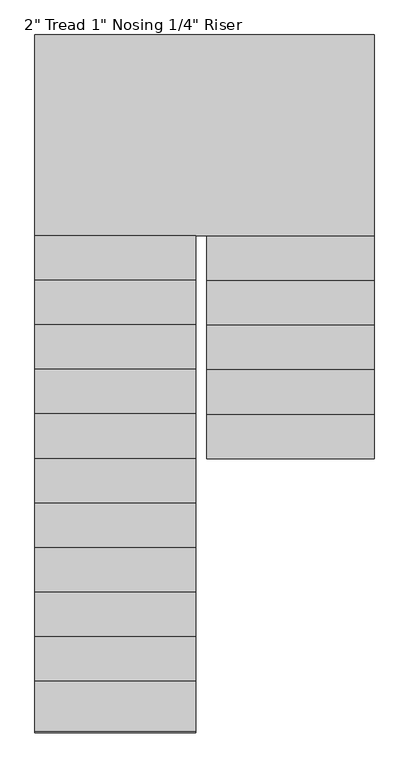
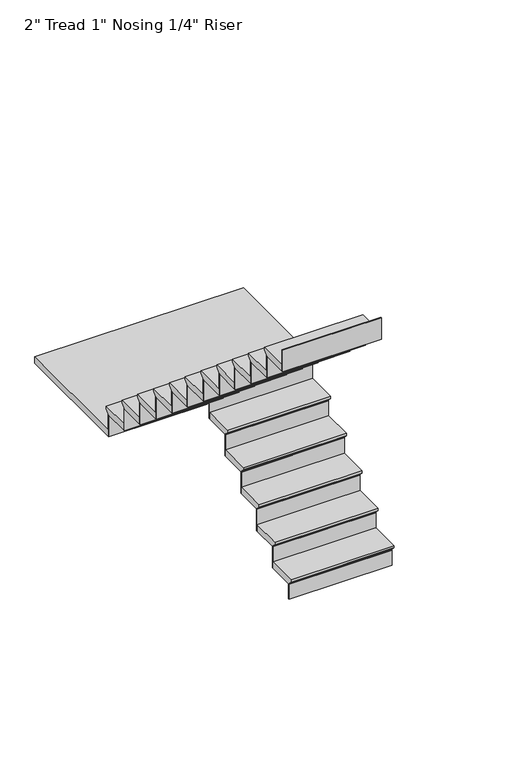
"""IFC4 building model written with IfcOpenShell, lengths in millimetres: stair flight geometry."""

from ifc_helpers import new_model, si_unit, origin, place, context, project, spatial, faceted_brep, source, transform, mapped, element, save


def stair_flight_8b765581(model_context):
    return source(origin(), model_context, "Body", "Brep", [
        faceted_brep([(-3749.597125, 2714.6319226, 33525.8833333), (-3749.597125, 2714.6319226, 33544.9333333), (-4512.2136682, 2714.6319226, 33544.9333333), (-4512.2136682, 2714.6319226, 33525.8833333), (-3749.597125, 2740.0319226, 33500.4833333), (-4512.2136682, 2740.0319226, 33500.4833333), (-3749.597125, 2943.2319226, 33544.9333333), (-4512.2136682, 2943.2319226, 33544.9333333), (-4512.2136682, 2740.0319226, 33494.1333333), (-4512.2136682, 2943.2319226, 33494.1333333), (-3749.597125, 2943.2319226, 33494.1333333), (-3749.597125, 2740.0319226, 33494.1333333)], [[[0, 1, 2, 3]], [[4, 0, 3, 5]], [[2, 1, 6, 7]], [[8, 9, 10, 11]], [[2, 7, 9, 8, 5, 3]], [[8, 11, 4, 5]], [[6, 1, 0, 4, 11, 10]], [[7, 6, 10, 9]]]),
        faceted_brep([(-3749.597125, 2740.0319226, 33494.1333333), (-3749.597125, 2740.0319226, 33375.6), (-3749.597125, 2746.3819226, 33375.6), (-3749.597125, 2746.3819226, 33494.1333333), (-4512.2136682, 2740.0319226, 33494.1333333), (-4512.2136682, 2746.3819226, 33494.1333333), (-4512.2136682, 2746.3819226, 33375.6), (-4512.2136682, 2740.0319226, 33375.6)], [[[0, 1, 2, 3]], [[4, 5, 6, 7]], [[1, 0, 4, 7]], [[2, 1, 7, 6]], [[3, 2, 6, 5]], [[0, 3, 5, 4]]]),
        faceted_brep([(-3749.597125, 2943.2319226, 33663.4666667), (-3749.597125, 2943.2319226, 33494.1333333), (-3749.597125, 2949.5819226, 33494.1333333), (-3749.597125, 2949.5819226, 33663.4666667), (-4512.2136682, 2943.2319226, 33663.4666667), (-4512.2136682, 2949.5819226, 33663.4666667), (-4512.2136682, 2949.5819226, 33494.1333333), (-4512.2136682, 2943.2319226, 33494.1333333)], [[[0, 1, 2, 3]], [[4, 5, 6, 7]], [[1, 0, 4, 7]], [[2, 1, 7, 6]], [[3, 2, 6, 5]], [[0, 3, 5, 4]]]),
        faceted_brep([(-4512.2136682, 2917.8319226, 33714.2666667), (-3749.597125, 2917.8319226, 33714.2666667), (-3749.597125, 3146.4319226, 33714.2666667), (-4512.2136682, 3146.4319226, 33714.2666667), (-4512.2136682, 2943.2319226, 33663.4666667), (-4512.2136682, 3146.4319226, 33663.4666667), (-3749.597125, 3146.4319226, 33663.4666667), (-3749.597125, 2943.2319226, 33663.4666667), (-4512.2136682, 2943.2319226, 33669.8166667), (-4512.2136682, 2917.8319226, 33695.2166667), (-3749.597125, 2943.2319226, 33669.8166667), (-3749.597125, 2917.8319226, 33695.2166667)], [[[0, 1, 2, 3]], [[4, 5, 6, 7]], [[0, 3, 5, 4, 8, 9]], [[4, 7, 10, 8]], [[2, 1, 11, 10, 7, 6]], [[3, 2, 6, 5]], [[11, 1, 0, 9]], [[10, 11, 9, 8]]]),
        faceted_brep([(-3749.597125, 3146.4319226, 33832.8), (-3749.597125, 3146.4319226, 33663.4666667), (-3749.597125, 3152.7819226, 33663.4666667), (-3749.597125, 3152.7819226, 33832.8), (-4512.2136682, 3146.4319226, 33832.8), (-4512.2136682, 3152.7819226, 33832.8), (-4512.2136682, 3152.7819226, 33663.4666667), (-4512.2136682, 3146.4319226, 33663.4666667)], [[[0, 1, 2, 3]], [[4, 5, 6, 7]], [[1, 0, 4, 7]], [[2, 1, 7, 6]], [[3, 2, 6, 5]], [[0, 3, 5, 4]]]),
        faceted_brep([(-4512.2136682, 3121.0319226, 33883.6), (-3749.597125, 3121.0319226, 33883.6), (-3749.597125, 3349.6319226, 33883.6), (-4512.2136682, 3349.6319226, 33883.6), (-4512.2136682, 3146.4319226, 33832.8), (-4512.2136682, 3349.6319226, 33832.8), (-3749.597125, 3349.6319226, 33832.8), (-3749.597125, 3146.4319226, 33832.8), (-4512.2136682, 3146.4319226, 33839.15), (-4512.2136682, 3121.0319226, 33864.55), (-3749.597125, 3146.4319226, 33839.15), (-3749.597125, 3121.0319226, 33864.55)], [[[0, 1, 2, 3]], [[4, 5, 6, 7]], [[0, 3, 5, 4, 8, 9]], [[4, 7, 10, 8]], [[2, 1, 11, 10, 7, 6]], [[3, 2, 6, 5]], [[11, 1, 0, 9]], [[10, 11, 9, 8]]]),
        faceted_brep([(-3749.597125, 3349.6319226, 34002.1333333), (-3749.597125, 3349.6319226, 33832.8), (-3749.597125, 3355.9819226, 33832.8), (-3749.597125, 3355.9819226, 34002.1333333), (-4512.2136682, 3349.6319226, 34002.1333333), (-4512.2136682, 3355.9819226, 34002.1333333), (-4512.2136682, 3355.9819226, 33832.8), (-4512.2136682, 3349.6319226, 33832.8)], [[[0, 1, 2, 3]], [[4, 5, 6, 7]], [[1, 0, 4, 7]], [[2, 1, 7, 6]], [[3, 2, 6, 5]], [[0, 3, 5, 4]]]),
        faceted_brep([(-4512.2136682, 3324.2319226, 34052.9333333), (-3749.597125, 3324.2319226, 34052.9333333), (-3749.597125, 3552.8319226, 34052.9333333), (-4512.2136682, 3552.8319226, 34052.9333333), (-4512.2136682, 3349.6319226, 34002.1333333), (-4512.2136682, 3552.8319226, 34002.1333333), (-3749.597125, 3552.8319226, 34002.1333333), (-3749.597125, 3349.6319226, 34002.1333333), (-4512.2136682, 3349.6319226, 34008.4833333), (-4512.2136682, 3324.2319226, 34033.8833333), (-3749.597125, 3349.6319226, 34008.4833333), (-3749.597125, 3324.2319226, 34033.8833333)], [[[0, 1, 2, 3]], [[4, 5, 6, 7]], [[0, 3, 5, 4, 8, 9]], [[4, 7, 10, 8]], [[2, 1, 11, 10, 7, 6]], [[3, 2, 6, 5]], [[11, 1, 0, 9]], [[10, 11, 9, 8]]]),
        faceted_brep([(-3749.597125, 3552.8319226, 34171.4666667), (-3749.597125, 3552.8319226, 34002.1333333), (-3749.597125, 3559.1819226, 34002.1333333), (-3749.597125, 3559.1819226, 34171.4666667), (-4512.2136682, 3552.8319226, 34171.4666667), (-4512.2136682, 3559.1819226, 34171.4666667), (-4512.2136682, 3559.1819226, 34002.1333333), (-4512.2136682, 3552.8319226, 34002.1333333)], [[[0, 1, 2, 3]], [[4, 5, 6, 7]], [[1, 0, 4, 7]], [[2, 1, 7, 6]], [[3, 2, 6, 5]], [[0, 3, 5, 4]]]),
        faceted_brep([(-4512.2136682, 3527.4319226, 34222.2666667), (-3749.597125, 3527.4319226, 34222.2666667), (-3749.597125, 3756.0319226, 34222.2666667), (-4512.2136682, 3756.0319226, 34222.2666667), (-4512.2136682, 3552.8319226, 34171.4666667), (-4512.2136682, 3756.0319226, 34171.4666667), (-3749.597125, 3756.0319226, 34171.4666667), (-3749.597125, 3552.8319226, 34171.4666667), (-4512.2136682, 3552.8319226, 34177.8166667), (-4512.2136682, 3527.4319226, 34203.2166667), (-3749.597125, 3552.8319226, 34177.8166667), (-3749.597125, 3527.4319226, 34203.2166667)], [[[0, 1, 2, 3]], [[4, 5, 6, 7]], [[0, 3, 5, 4, 8, 9]], [[4, 7, 10, 8]], [[2, 1, 11, 10, 7, 6]], [[3, 2, 6, 5]], [[11, 1, 0, 9]], [[10, 11, 9, 8]]]),
        faceted_brep([(-3749.597125, 3756.0319226, 34340.8), (-3749.597125, 3756.0319226, 34171.4666667), (-3749.597125, 3762.3819226, 34171.4666667), (-3749.597125, 3762.3819226, 34340.8), (-4512.2136682, 3756.0319226, 34340.8), (-4512.2136682, 3762.3819226, 34340.8), (-4512.2136682, 3762.3819226, 34171.4666667), (-4512.2136682, 3756.0319226, 34171.4666667)], [[[0, 1, 2, 3]], [[4, 5, 6, 7]], [[1, 0, 4, 7]], [[2, 1, 7, 6]], [[3, 2, 6, 5]], [[0, 3, 5, 4]]]),
        faceted_brep([(-4563.0136682, 3705.2319226, 34391.6), (-4563.0136682, 3730.6319226, 34391.6), (-3749.597125, 3730.6319226, 34391.6), (-3749.597125, 4645.0319226, 34391.6), (-5295.0246464, 4645.0319226, 34391.6), (-5295.0246464, 3705.2319226, 34391.6), (-4563.0136682, 3730.6319226, 34340.8), (-4563.0136682, 3705.2319226, 34340.8), (-5295.0246464, 3705.2319226, 34340.8), (-5295.0246464, 4645.0319226, 34340.8), (-3749.597125, 4645.0319226, 34340.8), (-3749.597125, 3756.0319226, 34340.8), (-4512.2136682, 3756.0319226, 34340.8), (-4512.2136682, 3730.6319226, 34340.8), (-4512.2136682, 3730.6319226, 34372.55), (-3749.597125, 3730.6319226, 34372.55), (-4512.2136682, 3756.0319226, 34347.15), (-3749.597125, 3756.0319226, 34347.15)], [[[0, 1, 2, 3, 4, 5]], [[6, 7, 8, 9, 10, 11, 12, 13]], [[1, 0, 7, 6]], [[2, 1, 6, 13, 14, 15]], [[13, 12, 16, 14]], [[12, 11, 17, 16]], [[3, 2, 15, 17, 11, 10]], [[4, 3, 10, 9]], [[5, 4, 9, 8]], [[0, 5, 8, 7]], [[17, 15, 14, 16]]]),
        faceted_brep([(-5295.0246464, 3705.2319226, 34510.1333333), (-5295.0246464, 3705.2319226, 34340.8), (-5295.0246464, 3698.8819226, 34340.8), (-5295.0246464, 3698.8819226, 34510.1333333), (-4563.0136682, 3705.2319226, 34510.1333333), (-4563.0136682, 3698.8819226, 34510.1333333), (-4563.0136682, 3698.8819226, 34340.8), (-4563.0136682, 3705.2319226, 34340.8)], [[[0, 1, 2, 3]], [[4, 5, 6, 7]], [[1, 0, 4, 7]], [[2, 1, 7, 6]], [[3, 2, 6, 5]], [[0, 3, 5, 4]]]),
        faceted_brep([(-4563.0136682, 3730.6319226, 34560.9333333), (-5295.0246464, 3730.6319226, 34560.9333333), (-5295.0246464, 3502.0319226, 34560.9333333), (-4563.0136682, 3502.0319226, 34560.9333333), (-4563.0136682, 3705.2319226, 34510.1333333), (-4563.0136682, 3502.0319226, 34510.1333333), (-5295.0246464, 3502.0319226, 34510.1333333), (-5295.0246464, 3705.2319226, 34510.1333333), (-4563.0136682, 3705.2319226, 34516.4833333), (-4563.0136682, 3730.6319226, 34541.8833333), (-5295.0246464, 3705.2319226, 34516.4833333), (-5295.0246464, 3730.6319226, 34541.8833333)], [[[0, 1, 2, 3]], [[4, 5, 6, 7]], [[0, 3, 5, 4, 8, 9]], [[4, 7, 10, 8]], [[2, 1, 11, 10, 7, 6]], [[3, 2, 6, 5]], [[11, 1, 0, 9]], [[10, 11, 9, 8]]]),
        faceted_brep([(-5295.0246464, 3502.0319226, 34679.4666667), (-5295.0246464, 3502.0319226, 34510.1333333), (-5295.0246464, 3495.6819226, 34510.1333333), (-5295.0246464, 3495.6819226, 34679.4666667), (-4563.0136682, 3502.0319226, 34679.4666667), (-4563.0136682, 3495.6819226, 34679.4666667), (-4563.0136682, 3495.6819226, 34510.1333333), (-4563.0136682, 3502.0319226, 34510.1333333)], [[[0, 1, 2, 3]], [[4, 5, 6, 7]], [[1, 0, 4, 7]], [[2, 1, 7, 6]], [[3, 2, 6, 5]], [[0, 3, 5, 4]]]),
        faceted_brep([(-4563.0136682, 3527.4319226, 34730.2666667), (-5295.0246464, 3527.4319226, 34730.2666667), (-5295.0246464, 3298.8319226, 34730.2666667), (-4563.0136682, 3298.8319226, 34730.2666667), (-4563.0136682, 3502.0319226, 34679.4666667), (-4563.0136682, 3298.8319226, 34679.4666667), (-5295.0246464, 3298.8319226, 34679.4666667), (-5295.0246464, 3502.0319226, 34679.4666667), (-4563.0136682, 3502.0319226, 34685.8166667), (-4563.0136682, 3527.4319226, 34711.2166667), (-5295.0246464, 3502.0319226, 34685.8166667), (-5295.0246464, 3527.4319226, 34711.2166667)], [[[0, 1, 2, 3]], [[4, 5, 6, 7]], [[0, 3, 5, 4, 8, 9]], [[4, 7, 10, 8]], [[2, 1, 11, 10, 7, 6]], [[3, 2, 6, 5]], [[11, 1, 0, 9]], [[10, 11, 9, 8]]]),
        faceted_brep([(-5295.0246464, 3298.8319226, 34848.8), (-5295.0246464, 3298.8319226, 34679.4666667), (-5295.0246464, 3292.4819226, 34679.4666667), (-5295.0246464, 3292.4819226, 34848.8), (-4563.0136682, 3298.8319226, 34848.8), (-4563.0136682, 3292.4819226, 34848.8), (-4563.0136682, 3292.4819226, 34679.4666667), (-4563.0136682, 3298.8319226, 34679.4666667)], [[[0, 1, 2, 3]], [[4, 5, 6, 7]], [[1, 0, 4, 7]], [[2, 1, 7, 6]], [[3, 2, 6, 5]], [[0, 3, 5, 4]]]),
        faceted_brep([(-4563.0136682, 3324.2319226, 34899.6), (-5295.0246464, 3324.2319226, 34899.6), (-5295.0246464, 3095.6319226, 34899.6), (-4563.0136682, 3095.6319226, 34899.6), (-4563.0136682, 3298.8319226, 34848.8), (-4563.0136682, 3095.6319226, 34848.8), (-5295.0246464, 3095.6319226, 34848.8), (-5295.0246464, 3298.8319226, 34848.8), (-4563.0136682, 3298.8319226, 34855.15), (-4563.0136682, 3324.2319226, 34880.55), (-5295.0246464, 3298.8319226, 34855.15), (-5295.0246464, 3324.2319226, 34880.55)], [[[0, 1, 2, 3]], [[4, 5, 6, 7]], [[0, 3, 5, 4, 8, 9]], [[4, 7, 10, 8]], [[2, 1, 11, 10, 7, 6]], [[3, 2, 6, 5]], [[11, 1, 0, 9]], [[10, 11, 9, 8]]]),
        faceted_brep([(-5295.0246464, 3095.6319226, 35018.1333333), (-5295.0246464, 3095.6319226, 34848.8), (-5295.0246464, 3089.2819226, 34848.8), (-5295.0246464, 3089.2819226, 35018.1333333), (-4563.0136682, 3095.6319226, 35018.1333333), (-4563.0136682, 3089.2819226, 35018.1333333), (-4563.0136682, 3089.2819226, 34848.8), (-4563.0136682, 3095.6319226, 34848.8)], [[[0, 1, 2, 3]], [[4, 5, 6, 7]], [[1, 0, 4, 7]], [[2, 1, 7, 6]], [[3, 2, 6, 5]], [[0, 3, 5, 4]]]),
        faceted_brep([(-4563.0136682, 3121.0319226, 35068.9333333), (-5295.0246464, 3121.0319226, 35068.9333333), (-5295.0246464, 2892.4319226, 35068.9333333), (-4563.0136682, 2892.4319226, 35068.9333333), (-4563.0136682, 3095.6319226, 35018.1333333), (-4563.0136682, 2892.4319226, 35018.1333333), (-5295.0246464, 2892.4319226, 35018.1333333), (-5295.0246464, 3095.6319226, 35018.1333333), (-4563.0136682, 3095.6319226, 35024.4833333), (-4563.0136682, 3121.0319226, 35049.8833333), (-5295.0246464, 3095.6319226, 35024.4833333), (-5295.0246464, 3121.0319226, 35049.8833333)], [[[0, 1, 2, 3]], [[4, 5, 6, 7]], [[0, 3, 5, 4, 8, 9]], [[4, 7, 10, 8]], [[2, 1, 11, 10, 7, 6]], [[3, 2, 6, 5]], [[11, 1, 0, 9]], [[10, 11, 9, 8]]]),
        faceted_brep([(-5295.0246464, 2892.4319226, 35187.4666667), (-5295.0246464, 2892.4319226, 35018.1333333), (-5295.0246464, 2886.0819226, 35018.1333333), (-5295.0246464, 2886.0819226, 35187.4666667), (-4563.0136682, 2892.4319226, 35187.4666667), (-4563.0136682, 2886.0819226, 35187.4666667), (-4563.0136682, 2886.0819226, 35018.1333333), (-4563.0136682, 2892.4319226, 35018.1333333)], [[[0, 1, 2, 3]], [[4, 5, 6, 7]], [[1, 0, 4, 7]], [[2, 1, 7, 6]], [[3, 2, 6, 5]], [[0, 3, 5, 4]]]),
        faceted_brep([(-4563.0136682, 2917.8319226, 35238.2666667), (-5295.0246464, 2917.8319226, 35238.2666667), (-5295.0246464, 2689.2319226, 35238.2666667), (-4563.0136682, 2689.2319226, 35238.2666667), (-4563.0136682, 2892.4319226, 35187.4666667), (-4563.0136682, 2689.2319226, 35187.4666667), (-5295.0246464, 2689.2319226, 35187.4666667), (-5295.0246464, 2892.4319226, 35187.4666667), (-4563.0136682, 2892.4319226, 35193.8166667), (-4563.0136682, 2917.8319226, 35219.2166667), (-5295.0246464, 2892.4319226, 35193.8166667), (-5295.0246464, 2917.8319226, 35219.2166667)], [[[0, 1, 2, 3]], [[4, 5, 6, 7]], [[0, 3, 5, 4, 8, 9]], [[4, 7, 10, 8]], [[2, 1, 11, 10, 7, 6]], [[3, 2, 6, 5]], [[11, 1, 0, 9]], [[10, 11, 9, 8]]]),
        faceted_brep([(-5295.0246464, 2689.2319226, 35356.8), (-5295.0246464, 2689.2319226, 35187.4666667), (-5295.0246464, 2682.8819226, 35187.4666667), (-5295.0246464, 2682.8819226, 35356.8), (-4563.0136682, 2689.2319226, 35356.8), (-4563.0136682, 2682.8819226, 35356.8), (-4563.0136682, 2682.8819226, 35187.4666667), (-4563.0136682, 2689.2319226, 35187.4666667)], [[[0, 1, 2, 3]], [[4, 5, 6, 7]], [[1, 0, 4, 7]], [[2, 1, 7, 6]], [[3, 2, 6, 5]], [[0, 3, 5, 4]]]),
        faceted_brep([(-4563.0136682, 2714.6319226, 35407.6), (-5295.0246464, 2714.6319226, 35407.6), (-5295.0246464, 2486.0319226, 35407.6), (-4563.0136682, 2486.0319226, 35407.6), (-4563.0136682, 2689.2319226, 35356.8), (-4563.0136682, 2486.0319226, 35356.8), (-5295.0246464, 2486.0319226, 35356.8), (-5295.0246464, 2689.2319226, 35356.8), (-4563.0136682, 2689.2319226, 35363.15), (-4563.0136682, 2714.6319226, 35388.55), (-5295.0246464, 2689.2319226, 35363.15), (-5295.0246464, 2714.6319226, 35388.55)], [[[0, 1, 2, 3]], [[4, 5, 6, 7]], [[0, 3, 5, 4, 8, 9]], [[4, 7, 10, 8]], [[2, 1, 11, 10, 7, 6]], [[3, 2, 6, 5]], [[11, 1, 0, 9]], [[10, 11, 9, 8]]]),
        faceted_brep([(-5295.0246464, 2486.0319226, 35526.1333333), (-5295.0246464, 2486.0319226, 35356.8), (-5295.0246464, 2479.6819226, 35356.8), (-5295.0246464, 2479.6819226, 35526.1333333), (-4563.0136682, 2486.0319226, 35526.1333333), (-4563.0136682, 2479.6819226, 35526.1333333), (-4563.0136682, 2479.6819226, 35356.8), (-4563.0136682, 2486.0319226, 35356.8)], [[[0, 1, 2, 3]], [[4, 5, 6, 7]], [[1, 0, 4, 7]], [[2, 1, 7, 6]], [[3, 2, 6, 5]], [[0, 3, 5, 4]]]),
        faceted_brep([(-4563.0136682, 2511.4319226, 35576.9333333), (-5295.0246464, 2511.4319226, 35576.9333333), (-5295.0246464, 2282.8319226, 35576.9333333), (-4563.0136682, 2282.8319226, 35576.9333333), (-4563.0136682, 2486.0319226, 35526.1333333), (-4563.0136682, 2282.8319226, 35526.1333333), (-5295.0246464, 2282.8319226, 35526.1333333), (-5295.0246464, 2486.0319226, 35526.1333333), (-4563.0136682, 2486.0319226, 35532.4833333), (-4563.0136682, 2511.4319226, 35557.8833333), (-5295.0246464, 2486.0319226, 35532.4833333), (-5295.0246464, 2511.4319226, 35557.8833333)], [[[0, 1, 2, 3]], [[4, 5, 6, 7]], [[0, 3, 5, 4, 8, 9]], [[4, 7, 10, 8]], [[2, 1, 11, 10, 7, 6]], [[3, 2, 6, 5]], [[11, 1, 0, 9]], [[10, 11, 9, 8]]]),
        faceted_brep([(-5295.0246464, 2282.8319226, 35695.4666667), (-5295.0246464, 2282.8319226, 35526.1333333), (-5295.0246464, 2276.4819226, 35526.1333333), (-5295.0246464, 2276.4819226, 35695.4666667), (-4563.0136682, 2282.8319226, 35695.4666667), (-4563.0136682, 2276.4819226, 35695.4666667), (-4563.0136682, 2276.4819226, 35526.1333333), (-4563.0136682, 2282.8319226, 35526.1333333)], [[[0, 1, 2, 3]], [[4, 5, 6, 7]], [[1, 0, 4, 7]], [[2, 1, 7, 6]], [[3, 2, 6, 5]], [[0, 3, 5, 4]]]),
        faceted_brep([(-4563.0136682, 2308.2319226, 35746.2666667), (-5295.0246464, 2308.2319226, 35746.2666667), (-5295.0246464, 2079.6319226, 35746.2666667), (-4563.0136682, 2079.6319226, 35746.2666667), (-4563.0136682, 2282.8319226, 35695.4666667), (-4563.0136682, 2079.6319226, 35695.4666667), (-5295.0246464, 2079.6319226, 35695.4666667), (-5295.0246464, 2282.8319226, 35695.4666667), (-4563.0136682, 2282.8319226, 35701.8166667), (-4563.0136682, 2308.2319226, 35727.2166667), (-5295.0246464, 2282.8319226, 35701.8166667), (-5295.0246464, 2308.2319226, 35727.2166667)], [[[0, 1, 2, 3]], [[4, 5, 6, 7]], [[0, 3, 5, 4, 8, 9]], [[4, 7, 10, 8]], [[2, 1, 11, 10, 7, 6]], [[3, 2, 6, 5]], [[11, 1, 0, 9]], [[10, 11, 9, 8]]]),
        faceted_brep([(-5295.0246464, 2079.6319226, 35864.8), (-5295.0246464, 2079.6319226, 35695.4666667), (-5295.0246464, 2073.2819226, 35695.4666667), (-5295.0246464, 2073.2819226, 35864.8), (-4563.0136682, 2079.6319226, 35864.8), (-4563.0136682, 2073.2819226, 35864.8), (-4563.0136682, 2073.2819226, 35695.4666667), (-4563.0136682, 2079.6319226, 35695.4666667)], [[[0, 1, 2, 3]], [[4, 5, 6, 7]], [[1, 0, 4, 7]], [[2, 1, 7, 6]], [[3, 2, 6, 5]], [[0, 3, 5, 4]]]),
        faceted_brep([(-4563.0136682, 2105.0319226, 35915.6), (-5295.0246464, 2105.0319226, 35915.6), (-5295.0246464, 1876.4319226, 35915.6), (-4563.0136682, 1876.4319226, 35915.6), (-4563.0136682, 2079.6319226, 35864.8), (-4563.0136682, 1876.4319226, 35864.8), (-5295.0246464, 1876.4319226, 35864.8), (-5295.0246464, 2079.6319226, 35864.8), (-4563.0136682, 2079.6319226, 35871.15), (-4563.0136682, 2105.0319226, 35896.55), (-5295.0246464, 2079.6319226, 35871.15), (-5295.0246464, 2105.0319226, 35896.55)], [[[0, 1, 2, 3]], [[4, 5, 6, 7]], [[0, 3, 5, 4, 8, 9]], [[4, 7, 10, 8]], [[2, 1, 11, 10, 7, 6]], [[3, 2, 6, 5]], [[11, 1, 0, 9]], [[10, 11, 9, 8]]]),
        faceted_brep([(-5295.0246464, 1876.4319226, 36034.1333333), (-5295.0246464, 1876.4319226, 35864.8), (-5295.0246464, 1870.0819226, 35864.8), (-5295.0246464, 1870.0819226, 36034.1333333), (-4563.0136682, 1876.4319226, 36034.1333333), (-4563.0136682, 1870.0819226, 36034.1333333), (-4563.0136682, 1870.0819226, 35864.8), (-4563.0136682, 1876.4319226, 35864.8)], [[[0, 1, 2, 3]], [[4, 5, 6, 7]], [[1, 0, 4, 7]], [[2, 1, 7, 6]], [[3, 2, 6, 5]], [[0, 3, 5, 4]]]),
        faceted_brep([(-4563.0136682, 1901.8319226, 36084.9333333), (-5295.0246464, 1901.8319226, 36084.9333333), (-5295.0246464, 1673.2319226, 36084.9333333), (-4563.0136682, 1673.2319226, 36084.9333333), (-4563.0136682, 1876.4319226, 36034.1333333), (-4563.0136682, 1673.2319226, 36034.1333333), (-5295.0246464, 1673.2319226, 36034.1333333), (-5295.0246464, 1876.4319226, 36034.1333333), (-4563.0136682, 1876.4319226, 36040.4833333), (-4563.0136682, 1901.8319226, 36065.8833333), (-5295.0246464, 1876.4319226, 36040.4833333), (-5295.0246464, 1901.8319226, 36065.8833333)], [[[0, 1, 2, 3]], [[4, 5, 6, 7]], [[0, 3, 5, 4, 8, 9]], [[4, 7, 10, 8]], [[2, 1, 11, 10, 7, 6]], [[3, 2, 6, 5]], [[11, 1, 0, 9]], [[10, 11, 9, 8]]]),
        faceted_brep([(-5295.0246464, 1673.2319226, 36203.4666667), (-5295.0246464, 1673.2319226, 36034.1333333), (-5295.0246464, 1666.8819226, 36034.1333333), (-5295.0246464, 1666.8819226, 36203.4666667), (-4563.0136682, 1673.2319226, 36203.4666667), (-4563.0136682, 1666.8819226, 36203.4666667), (-4563.0136682, 1666.8819226, 36034.1333333), (-4563.0136682, 1673.2319226, 36034.1333333)], [[[0, 1, 2, 3]], [[4, 5, 6, 7]], [[1, 0, 4, 7]], [[2, 1, 7, 6]], [[3, 2, 6, 5]], [[0, 3, 5, 4]]]),
        faceted_brep([(-4563.0136682, 1698.6319226, 36254.2666667), (-5295.0246464, 1698.6319226, 36254.2666667), (-5295.0246464, 1470.0319226, 36254.2666667), (-4563.0136682, 1470.0319226, 36254.2666667), (-4563.0136682, 1673.2319226, 36203.4666667), (-4563.0136682, 1470.0319226, 36203.4666667), (-5295.0246464, 1470.0319226, 36203.4666667), (-5295.0246464, 1673.2319226, 36203.4666667), (-4563.0136682, 1673.2319226, 36209.8166667), (-4563.0136682, 1698.6319226, 36235.2166667), (-5295.0246464, 1673.2319226, 36209.8166667), (-5295.0246464, 1698.6319226, 36235.2166667)], [[[0, 1, 2, 3]], [[4, 5, 6, 7]], [[0, 3, 5, 4, 8, 9]], [[4, 7, 10, 8]], [[2, 1, 11, 10, 7, 6]], [[3, 2, 6, 5]], [[11, 1, 0, 9]], [[10, 11, 9, 8]]]),
        faceted_brep([(-5295.0246464, 1470.0319226, 36372.8), (-5295.0246464, 1470.0319226, 36203.4666667), (-5295.0246464, 1463.6819226, 36203.4666667), (-5295.0246464, 1463.6819226, 36372.8), (-4563.0136682, 1470.0319226, 36372.8), (-4563.0136682, 1463.6819226, 36372.8), (-4563.0136682, 1463.6819226, 36203.4666667), (-4563.0136682, 1470.0319226, 36203.4666667)], [[[0, 1, 2, 3]], [[4, 5, 6, 7]], [[1, 0, 4, 7]], [[2, 1, 7, 6]], [[3, 2, 6, 5]], [[0, 3, 5, 4]]]),
    ])


if __name__ == "__main__":
    model = new_model("IFC4")
    model_context = context("Model", 3, world=origin())
    ifc_project = project(units=[si_unit("LENGTHUNIT", "METRE", prefix="MILLI")], contexts=[model_context])
    site = spatial("IfcSite", under=ifc_project)
    building = spatial("IfcBuilding", under=site)
    placement = place(None, origin())
    stair_flight_shape = stair_flight_8b765581(model_context)
    element("IfcStairFlight", 1, ObjectType="2\" Tread 1\" Nosing 1/4\" Riser", at=placement, inside=building, context=model_context, shape_type="MappedRepresentation", body=[
        mapped(stair_flight_shape, transform((0.0, 0.0, 0.0), x_axis=(1.0, 0.0, 0.0), y_axis=(0.0, 1.0, 0.0), z_axis=(0.0, 0.0, 1.0))),
    ])
    save(model, "model.ifc")
